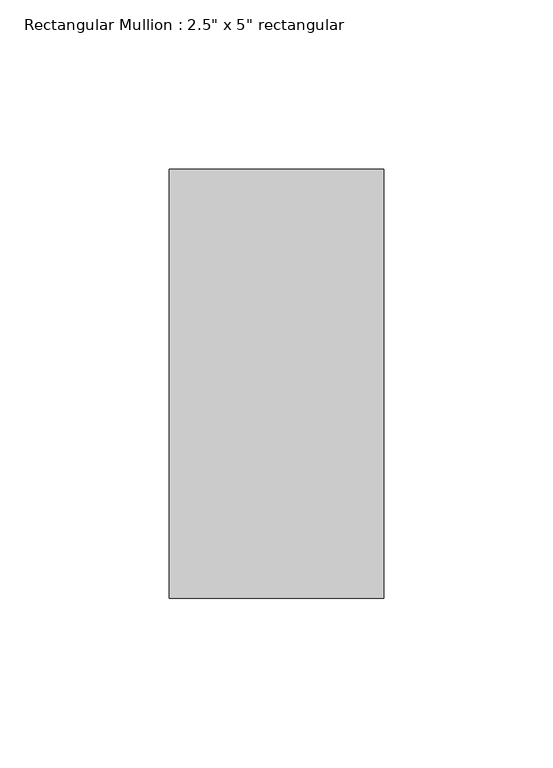
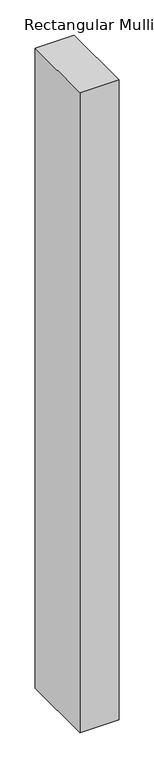
"""IFC4 building model written with IfcOpenShell, lengths in millimetres: member geometry."""

from ifc_helpers import new_model, si_unit, frame, origin, place, context, project, spatial, polyline, outline, extrude, source, transform, mapped, element, save


def member_f5e9651f(model_context):
    return source(origin(), model_context, "Body", "SweptSolid", [
        extrude(outline(polyline([(0.0, 63.5), (0.0, -63.5), (-63.5, -63.5), (-63.5, 63.5), (0.0, 63.5)])), frame((0.0, 0.0, -1104.8999998), z_axis=(0.0, 0.0, 1.0), x_axis=(1.0, 0.0, 0.0)), (0.0, 0.0, 1.0), 1104.8999998),
    ])


if __name__ == "__main__":
    model = new_model("IFC4")
    model_context = context("Model", 3, world=origin())
    ifc_project = project(units=[si_unit("LENGTHUNIT", "METRE", prefix="MILLI")], contexts=[model_context])
    site = spatial("IfcSite", under=ifc_project)
    building = spatial("IfcBuilding", under=site)
    placement = place(None, origin())
    member_shape = member_f5e9651f(model_context)
    element("IfcMember", 1, ObjectType="Rectangular Mullion : 2.5\" x 5\" rectangular", at=placement, inside=building, context=model_context, shape_type="MappedRepresentation", body=[
        mapped(member_shape, transform((0.0, 0.0, 0.0), x_axis=(1.0, 0.0, 0.0), y_axis=(0.0, 1.0, 0.0), z_axis=(0.0, 0.0, 1.0))),
    ])
    save(model, "model.ifc")

# Revit data of these elements
# Type "Rectangular Mullion : 2.5\" x 5\" rectangular"
#   built-in parameter 1007304 = 0.416667 (stored number, unit not read)
#   built-in parameter 1007301 = 0.104167 (stored number, unit not read)
#   built-in parameter 1007300 = 0.104167 (stored number, unit not read)
# Element 1 (IfcMember, "Rectangular Mullion : 2.5\" x 5\" rectangular")
#   Materials on its faces: "Aluminum"
# Materials
#   "Aluminum": class "Metal", colour RGB 247 247 247, transparency 0, Description = "Aluminum 6061", Cost = 0
